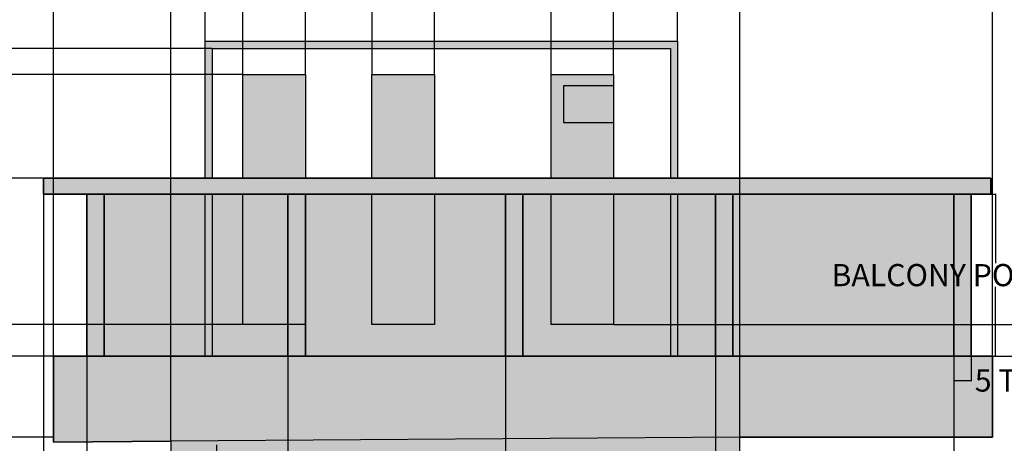
# Model space of a CAD drawing. Units: inches. Extents: x -655 to 499, y 20 to 616.
# Tile 3 of 7: x -409 to -137, y 248 to 365. Entities that reach past the tile are written whole.
import ezdxf

# ---------------------------------------------------------------- set-up
doc = ezdxf.new("R2010")
doc.units = ezdxf.units.IN
doc.header["$MEASUREMENT"] = 0
for name, color, linetype, lineweight in [('A-ANNO-DIMS', 2, 'Continuous', 18), ('A-ELEV', 7, 'Continuous', 35), ('A-ELEV-PATT', 9, 'Continuous', 13), ('A-GLAZ', 3, 'Continuous', 25)]:
    doc.layers.add(name, color=color, linetype=linetype, lineweight=lineweight)
doc.styles.get("Standard").update_dxf_attribs({"font": 'arial.ttf'})
doc.dimstyles.get("Standard").update_dxf_attribs({"dimtxt": 6.125, "dimasz": 0.18, "dimexe": 0.18, "dimexo": 0.0625, "dimgap": 0.09, "dimtad": 0, "dimtih": 1, "dimtoh": 1, "dimdec": 4, "dimzin": 0, "dimdsep": 46, "dimlunit": 4, "dimtxsty": 'Standard', "dimcen": 0.09, "dimadec": 0, "dimazin": 0, "dimtfac": 1, "dimtdec": 4, "dimtofl": 0, "dimtmove": 0, "dimatfit": 3, "dimfxl": 1, "dimtolj": 1, "dimtzin": 0, "dimarcsym": 0})

# ---------------------------------------------------------------- blocks, each defined once
blk = doc.blocks.new('BALCONY-POST')
for p, q in [((0, 0), (0, 44.79)), ((0, 44.79), (0, 44.79)), ((0, 44.79), (4.81, 44.79)), ((4.81, 44.79), (4.81, 0))]:
    blk.add_line(p, q)
blk = doc.blocks.new('*D4')
at = {"layer": 'A-ANNO-DIMS', "color": 0, "lineweight": -2, "transparency": 16777216}
for p, q in [((-145.9, 317.05), (-139.06, 317.05)), ((-139.24, 316.87), (-139.24, 297.92)), ((-139.24, 272.44), (-139.24, 291.4)), ((-145.9, 272.26), (-139.06, 272.26))]:
    blk.add_line(p, q, dxfattribs=at)
at = {"layer": 'A-ANNO-DIMS', "color": 0, "transparency": 16777216}
for points in [[(-139.27, 316.87), (-139.21, 316.87), (-139.24, 317.05)], [(-139.27, 272.44), (-139.21, 272.44), (-139.24, 272.26)]]:
    blk.add_solid(points, dxfattribs=at)
at = {"layer": 'Defpoints', "color": 0, "transparency": 16777216}
for p in [(-145.96, 317.05), (-139.24, 317.05), (-145.96, 272.26)]:
    blk.add_point(p, dxfattribs=at)
at = {"layer": 'A-ANNO-DIMS', "color": 0, "transparency": 16777216, "insert": (-139.24, 294.66), "char_height": 6.125, "attachment_point": 5}
blk.add_mtext('\\A1;BALCONY POST 45 TYP.', dxfattribs=at)
blk = doc.blocks.new('*D5')
at = {"layer": 'A-ANNO-DIMS', "color": 0, "lineweight": -2, "transparency": 16777216}
for p, q in [((-150.77, 272.2), (-150.77, 265.36)), ((-145.96, 272.2), (-145.96, 265.36)), ((-150.59, 265.54), (-146.14, 265.54)), ((-145.96, 265.54), (-145.78, 265.54))]:
    blk.add_line(p, q, dxfattribs=at)
at = {"layer": 'A-ANNO-DIMS', "color": 0, "transparency": 16777216}
for points in [[(-150.59, 265.57), (-150.59, 265.51), (-150.77, 265.54)], [(-146.14, 265.57), (-146.14, 265.51), (-145.96, 265.54)]]:
    blk.add_solid(points, dxfattribs=at)
at = {"layer": 'Defpoints', "color": 0, "transparency": 16777216}
for p in [(-150.77, 272.26), (-145.96, 272.26), (-145.96, 265.54)]:
    blk.add_point(p, dxfattribs=at)
at = {"layer": 'A-ANNO-DIMS', "color": 0, "transparency": 16777216, "insert": (-133.16, 265.54), "char_height": 6.125, "attachment_point": 5}
blk.add_mtext('\\A1;5 TYP.', dxfattribs=at)
blk = doc.blocks.new('*D10')
at = {"layer": 'A-ANNO-DIMS', "color": 0, "lineweight": -2, "transparency": 16777216}
for p, q in [((434.11, 393.11), (434.11, 23.7)), ((-590.16, 75.57), (-590.16, 23.7)), ((-589.98, 23.88), (-90.54, 23.88)), ((433.93, 23.88), (-65.51, 23.88))]:
    blk.add_line(p, q, dxfattribs=at)
at = {"layer": 'A-ANNO-DIMS', "color": 0, "transparency": 16777216}
for points in [[(-589.98, 23.91), (-589.98, 23.85), (-590.16, 23.88)], [(433.93, 23.91), (433.93, 23.85), (434.11, 23.88)]]:
    blk.add_solid(points, dxfattribs=at)
at = {"layer": 'Defpoints', "color": 0, "transparency": 16777216}
for p in [(434.11, 393.17), (-590.16, 75.63), (434.11, 23.88)]:
    blk.add_point(p, dxfattribs=at)
at = {"layer": 'A-ANNO-DIMS', "color": 0, "transparency": 16777216, "insert": (-78.02, 23.88), "char_height": 6.125, "attachment_point": 5}
blk.add_mtext('\\A1;1024.3', dxfattribs=at)
blk = doc.blocks.new('*D17')
at = {"layer": 'A-ANNO-DIMS', "color": 0, "lineweight": -2, "transparency": 16777216}
for p, q in [((-399.38, 249.9), (-399.38, 611.71)), ((-399.2, 611.53), (-282.57, 611.53)), ((-140.23, 611.53), (-256.86, 611.53)), ((-140.05, 249.9), (-140.05, 611.71))]:
    blk.add_line(p, q, dxfattribs=at)
at = {"layer": 'A-ANNO-DIMS', "color": 0, "transparency": 16777216}
for points in [[(-399.2, 611.56), (-399.2, 611.5), (-399.38, 611.53)], [(-140.23, 611.56), (-140.23, 611.5), (-140.05, 611.53)]]:
    blk.add_solid(points, dxfattribs=at)
at = {"layer": 'Defpoints', "color": 0, "transparency": 16777216}
for p in [(-140.05, 611.53), (-399.38, 249.84), (-140.05, 249.84)]:
    blk.add_point(p, dxfattribs=at)
at = {"layer": 'A-ANNO-DIMS', "color": 0, "transparency": 16777216, "insert": (-269.71, 611.53), "char_height": 6.125, "attachment_point": 5}
blk.add_mtext('\\A1;259.33', dxfattribs=at)
blk = doc.blocks.new('*D21')
at = {"layer": 'A-ANNO-DIMS', "color": 0, "lineweight": -2, "transparency": 16777216}
for p, q in [((179.11, 559.78), (486.04, 559.78)), ((485.86, 559.6), (485.86, 320.92)), ((485.86, 75.81), (485.86, 314.49)), ((-590.1, 75.63), (486.04, 75.63))]:
    blk.add_line(p, q, dxfattribs=at)
at = {"layer": 'A-ANNO-DIMS', "color": 0, "transparency": 16777216}
for points in [[(485.83, 559.6), (485.89, 559.6), (485.86, 559.78)], [(485.83, 75.81), (485.89, 75.81), (485.86, 75.63)]]:
    blk.add_solid(points, dxfattribs=at)
at = {"layer": 'Defpoints', "color": 0, "transparency": 16777216}
for p in [(179.05, 559.78), (485.86, 559.78), (-590.16, 75.63)]:
    blk.add_point(p, dxfattribs=at)
at = {"layer": 'A-ANNO-DIMS', "color": 0, "transparency": 16777216, "insert": (485.86, 317.7), "char_height": 6.125, "attachment_point": 5}
blk.add_mtext('\\A1;484.15', dxfattribs=at)
blk = doc.blocks.new('*D25')
at = {"layer": 'A-ANNO-DIMS', "color": 0, "lineweight": -2, "transparency": 16777216}
for p, q in [((-399.44, 249.84), (-642.09, 249.84)), ((-641.91, 249.66), (-641.91, 177.41)), ((-641.91, 98.71), (-641.91, 170.97)), ((-367.01, 98.53), (-642.09, 98.53))]:
    blk.add_line(p, q, dxfattribs=at)
at = {"layer": 'A-ANNO-DIMS', "color": 0, "transparency": 16777216}
for points in [[(-641.94, 249.66), (-641.88, 249.66), (-641.91, 249.84)], [(-641.94, 98.71), (-641.88, 98.71), (-641.91, 98.53)]]:
    blk.add_solid(points, dxfattribs=at)
at = {"layer": 'Defpoints', "color": 0, "transparency": 16777216}
for p in [(-399.38, 249.84), (-641.91, 98.53), (-366.94, 98.53)]:
    blk.add_point(p, dxfattribs=at)
at = {"layer": 'A-ANNO-DIMS', "color": 0, "transparency": 16777216, "insert": (-641.91, 174.19), "char_height": 6.125, "attachment_point": 5}
blk.add_mtext('\\A1;151.3', dxfattribs=at)
blk = doc.blocks.new('*D26')
at = {"layer": 'A-ANNO-DIMS', "color": 0, "lineweight": -2, "transparency": 16777216}
for p, q in [((-355.49, 357.29), (-642.09, 357.29)), ((-641.91, 357.11), (-641.91, 317.99)), ((-641.91, 272.44), (-641.91, 311.56)), ((-355.49, 272.26), (-642.09, 272.26))]:
    blk.add_line(p, q, dxfattribs=at)
at = {"layer": 'A-ANNO-DIMS', "color": 0, "transparency": 16777216}
for points in [[(-641.94, 357.11), (-641.88, 357.11), (-641.91, 357.29)], [(-641.94, 272.44), (-641.88, 272.44), (-641.91, 272.26)]]:
    blk.add_solid(points, dxfattribs=at)
at = {"layer": 'Defpoints', "color": 0, "transparency": 16777216}
for p in [(-641.91, 357.29), (-355.43, 357.29), (-355.43, 272.26)]:
    blk.add_point(p, dxfattribs=at)
at = {"layer": 'A-ANNO-DIMS', "color": 0, "transparency": 16777216, "insert": (-641.91, 314.77), "char_height": 6.125, "attachment_point": 5}
blk.add_mtext('\\A1;85.02', dxfattribs=at)
blk = doc.blocks.new('*D27')
at = {"layer": 'A-ANNO-DIMS', "color": 0, "lineweight": -2, "transparency": 16777216}
for p, q in [((-357.43, 359.35), (-357.43, 611.71)), ((-357.25, 611.53), (-347.21, 611.53)), ((-347.03, 350.2), (-347.03, 611.71)), ((-347.03, 611.53), (-346.85, 611.53))]:
    blk.add_line(p, q, dxfattribs=at)
at = {"layer": 'A-ANNO-DIMS', "color": 0, "transparency": 16777216}
for points in [[(-357.25, 611.56), (-357.25, 611.5), (-357.43, 611.53)], [(-347.21, 611.56), (-347.21, 611.5), (-347.03, 611.53)]]:
    blk.add_solid(points, dxfattribs=at)
at = {"layer": 'Defpoints', "color": 0, "transparency": 16777216}
for p in [(-347.03, 611.53), (-357.43, 359.29), (-347.03, 350.13)]:
    blk.add_point(p, dxfattribs=at)
at = {"layer": 'A-ANNO-DIMS', "color": 0, "transparency": 16777216, "insert": (-334.32, 611.53), "char_height": 6.125, "attachment_point": 5}
blk.add_mtext('\\A1;10.395', dxfattribs=at)
blk = doc.blocks.new('*D28')
at = {"layer": 'A-ANNO-DIMS', "color": 0, "lineweight": -2, "transparency": 16777216}
for p, q in [((-347.03, 350.2), (-347.03, 611.71)), ((-346.85, 611.53), (-329.96, 611.53)), ((-329.78, 350.2), (-329.78, 611.71)), ((-329.78, 611.53), (-329.6, 611.53))]:
    blk.add_line(p, q, dxfattribs=at)
at = {"layer": 'A-ANNO-DIMS', "color": 0, "transparency": 16777216}
for points in [[(-346.85, 611.56), (-346.85, 611.5), (-347.03, 611.53)], [(-329.96, 611.56), (-329.96, 611.5), (-329.78, 611.53)]]:
    blk.add_solid(points, dxfattribs=at)
at = {"layer": 'Defpoints', "color": 0, "transparency": 16777216}
for p in [(-329.78, 611.53), (-347.03, 350.13), (-329.78, 350.13)]:
    blk.add_point(p, dxfattribs=at)
at = {"layer": 'A-ANNO-DIMS', "color": 0, "transparency": 16777216, "insert": (-319.44, 611.53), "char_height": 6.125, "attachment_point": 5}
blk.add_mtext('\\A1;17.25', dxfattribs=at)
blk = doc.blocks.new('*D29')
at = {"layer": 'A-ANNO-DIMS', "color": 0, "lineweight": -2, "transparency": 16777216}
for p, q in [((-329.78, 350.2), (-329.78, 611.71)), ((-329.6, 611.53), (-311.57, 611.53)), ((-311.39, 350.2), (-311.39, 611.71)), ((-311.39, 611.53), (-311.21, 611.53))]:
    blk.add_line(p, q, dxfattribs=at)
at = {"layer": 'A-ANNO-DIMS', "color": 0, "transparency": 16777216}
for points in [[(-329.6, 611.56), (-329.6, 611.5), (-329.78, 611.53)], [(-311.57, 611.56), (-311.57, 611.5), (-311.39, 611.53)]]:
    blk.add_solid(points, dxfattribs=at)
at = {"layer": 'Defpoints', "color": 0, "transparency": 16777216}
for p in [(-311.39, 611.53), (-329.78, 350.13), (-311.39, 350.13)]:
    blk.add_point(p, dxfattribs=at)
at = {"layer": 'A-ANNO-DIMS', "color": 0, "transparency": 16777216, "insert": (-298.73, 611.53), "char_height": 6.125, "attachment_point": 5}
blk.add_mtext('\\A1;18.392', dxfattribs=at)
blk = doc.blocks.new('*D30')
at = {"layer": 'A-ANNO-DIMS', "color": 0, "lineweight": -2, "transparency": 16777216}
for p, q in [((-311.39, 350.2), (-311.39, 611.71)), ((-311.21, 611.53), (-294.32, 611.53)), ((-294.14, 350.2), (-294.14, 611.71)), ((-294.14, 611.53), (-293.96, 611.53))]:
    blk.add_line(p, q, dxfattribs=at)
at = {"layer": 'A-ANNO-DIMS', "color": 0, "transparency": 16777216}
for points in [[(-311.21, 611.56), (-311.21, 611.5), (-311.39, 611.53)], [(-294.32, 611.56), (-294.32, 611.5), (-294.14, 611.53)]]:
    blk.add_solid(points, dxfattribs=at)
at = {"layer": 'Defpoints', "color": 0, "transparency": 16777216}
for p in [(-294.14, 611.53), (-311.39, 350.13), (-294.14, 350.13)]:
    blk.add_point(p, dxfattribs=at)
at = {"layer": 'A-ANNO-DIMS', "color": 0, "transparency": 16777216, "insert": (-283.8, 611.53), "char_height": 6.125, "attachment_point": 5}
blk.add_mtext('\\A1;17.25', dxfattribs=at)
blk = doc.blocks.new('*D31')
at = {"layer": 'A-ANNO-DIMS', "color": 0, "lineweight": -2, "transparency": 16777216}
for p, q in [((-294.14, 350.2), (-294.14, 611.71)), ((-293.96, 611.53), (-290.86, 611.53)), ((-262.12, 611.53), (-265.21, 611.53)), ((-261.94, 350.2), (-261.94, 611.71))]:
    blk.add_line(p, q, dxfattribs=at)
at = {"layer": 'A-ANNO-DIMS', "color": 0, "transparency": 16777216}
for points in [[(-293.96, 611.56), (-293.96, 611.5), (-294.14, 611.53)], [(-262.12, 611.56), (-262.12, 611.5), (-261.94, 611.53)]]:
    blk.add_solid(points, dxfattribs=at)
at = {"layer": 'Defpoints', "color": 0, "transparency": 16777216}
for p in [(-261.94, 611.53), (-294.14, 350.13), (-261.94, 350.13)]:
    blk.add_point(p, dxfattribs=at)
at = {"layer": 'A-ANNO-DIMS', "color": 0, "transparency": 16777216, "insert": (-278.04, 611.53), "char_height": 6.125, "attachment_point": 5}
blk.add_mtext('\\A1;32.205', dxfattribs=at)
blk = doc.blocks.new('*D32')
at = {"layer": 'A-ANNO-DIMS', "color": 0, "lineweight": -2, "transparency": 16777216}
for p, q in [((-261.94, 350.2), (-261.94, 611.71)), ((-261.76, 611.53), (-244.87, 611.53)), ((-244.69, 350.2), (-244.69, 611.71)), ((-244.69, 611.53), (-244.51, 611.53))]:
    blk.add_line(p, q, dxfattribs=at)
at = {"layer": 'A-ANNO-DIMS', "color": 0, "transparency": 16777216}
for points in [[(-261.76, 611.56), (-261.76, 611.5), (-261.94, 611.53)], [(-244.87, 611.56), (-244.87, 611.5), (-244.69, 611.53)]]:
    blk.add_solid(points, dxfattribs=at)
at = {"layer": 'Defpoints', "color": 0, "transparency": 16777216}
for p in [(-244.69, 611.53), (-261.94, 350.13), (-244.69, 350.13)]:
    blk.add_point(p, dxfattribs=at)
at = {"layer": 'A-ANNO-DIMS', "color": 0, "transparency": 16777216, "insert": (-234.35, 611.53), "char_height": 6.125, "attachment_point": 5}
blk.add_mtext('\\A1;17.25', dxfattribs=at)
blk = doc.blocks.new('*D33')
at = {"layer": 'A-ANNO-DIMS', "color": 0, "lineweight": -2, "transparency": 16777216}
for p, q in [((-244.69, 350.2), (-244.69, 611.71)), ((-244.51, 611.53), (-227.19, 611.53)), ((-227.01, 359.35), (-227.01, 611.71)), ((-227.01, 611.53), (-226.83, 611.53))]:
    blk.add_line(p, q, dxfattribs=at)
at = {"layer": 'A-ANNO-DIMS', "color": 0, "transparency": 16777216}
for points in [[(-244.51, 611.56), (-244.51, 611.5), (-244.69, 611.53)], [(-227.19, 611.56), (-227.19, 611.5), (-227.01, 611.53)]]:
    blk.add_solid(points, dxfattribs=at)
at = {"layer": 'Defpoints', "color": 0, "transparency": 16777216}
for p in [(-227.01, 611.53), (-227.01, 359.29), (-244.69, 350.13)]:
    blk.add_point(p, dxfattribs=at)
at = {"layer": 'A-ANNO-DIMS', "color": 0, "transparency": 16777216, "insert": (-214.31, 611.53), "char_height": 6.125, "attachment_point": 5}
blk.add_mtext('\\A1;17.677', dxfattribs=at)
blk = doc.blocks.new('*D34')
at = {"layer": 'A-ANNO-DIMS', "color": 0, "lineweight": -2, "transparency": 16777216}
for p, q in [((-347.1, 350.13), (-642.09, 350.13)), ((-641.91, 349.95), (-641.91, 318.77)), ((-641.91, 281.15), (-641.91, 312.33)), ((-347.1, 280.97), (-642.09, 280.97))]:
    blk.add_line(p, q, dxfattribs=at)
at = {"layer": 'A-ANNO-DIMS', "color": 0, "transparency": 16777216}
for points in [[(-641.94, 349.95), (-641.88, 349.95), (-641.91, 350.13)], [(-641.94, 281.15), (-641.88, 281.15), (-641.91, 280.97)]]:
    blk.add_solid(points, dxfattribs=at)
at = {"layer": 'Defpoints', "color": 0, "transparency": 16777216}
for p in [(-347.03, 350.13), (-641.91, 280.97), (-347.03, 280.97)]:
    blk.add_point(p, dxfattribs=at)
at = {"layer": 'A-ANNO-DIMS', "color": 0, "transparency": 16777216, "insert": (-641.91, 315.55), "char_height": 6.125, "attachment_point": 5}
blk.add_mtext('\\A1;69.17', dxfattribs=at)
blk = doc.blocks.new('*D35')
at = {"layer": 'A-ANNO-DIMS', "color": 0, "lineweight": -2, "transparency": 16777216}
for p, q in [((-244.62, 280.97), (486.04, 280.97)), ((485.86, 280.79), (485.86, 279.83)), ((-226.95, 272.26), (486.04, 272.26)), ((485.86, 272.44), (485.86, 273.4))]:
    blk.add_line(p, q, dxfattribs=at)
at = {"layer": 'A-ANNO-DIMS', "color": 0, "transparency": 16777216}
for points in [[(485.83, 280.79), (485.89, 280.79), (485.86, 280.97)], [(485.83, 272.44), (485.89, 272.44), (485.86, 272.26)]]:
    blk.add_solid(points, dxfattribs=at)
at = {"layer": 'Defpoints', "color": 0, "transparency": 16777216}
for p in [(-244.69, 280.97), (-227.01, 272.26), (485.86, 272.26)]:
    blk.add_point(p, dxfattribs=at)
at = {"layer": 'A-ANNO-DIMS', "color": 0, "transparency": 16777216, "insert": (485.86, 276.61), "char_height": 6.125, "attachment_point": 5}
blk.add_mtext('\\A1;8.706', dxfattribs=at)
blk = doc.blocks.new('*D36')
at = {"layer": 'A-ANNO-DIMS', "color": 0, "lineweight": -2, "transparency": 16777216}
for p, q in [((-399.44, 272.26), (-642.09, 272.26)), ((-641.91, 272.08), (-641.91, 264.22)), ((-641.91, 250.02), (-641.91, 257.89)), ((-399.44, 249.84), (-642.09, 249.84))]:
    blk.add_line(p, q, dxfattribs=at)
at = {"layer": 'A-ANNO-DIMS', "color": 0, "transparency": 16777216}
for points in [[(-641.94, 272.08), (-641.88, 272.08), (-641.91, 272.26)], [(-641.94, 250.02), (-641.88, 250.02), (-641.91, 249.84)]]:
    blk.add_solid(points, dxfattribs=at)
at = {"layer": 'Defpoints', "color": 0, "transparency": 16777216}
for p in [(-641.91, 272.26), (-399.38, 272.26), (-399.38, 249.84)]:
    blk.add_point(p, dxfattribs=at)
at = {"layer": 'A-ANNO-DIMS', "color": 0, "transparency": 16777216, "insert": (-641.91, 261.05), "char_height": 6.125, "attachment_point": 5}
blk.add_mtext('\\A1;22.42', dxfattribs=at)
blk = doc.blocks.new('*D37')
at = {"layer": 'A-ANNO-DIMS', "color": 0, "lineweight": -2, "transparency": 16777216}
for p, q in [((-402.14, 321.49), (-642.09, 321.49)), ((-641.91, 321.31), (-641.91, 300.09)), ((-641.91, 272.44), (-641.91, 293.66)), ((-399.44, 272.26), (-642.09, 272.26))]:
    blk.add_line(p, q, dxfattribs=at)
at = {"layer": 'A-ANNO-DIMS', "color": 0, "transparency": 16777216}
for points in [[(-641.94, 321.31), (-641.88, 321.31), (-641.91, 321.49)], [(-641.94, 272.44), (-641.88, 272.44), (-641.91, 272.26)]]:
    blk.add_solid(points, dxfattribs=at)
at = {"layer": 'Defpoints', "color": 0, "transparency": 16777216}
for p in [(-641.91, 321.49), (-402.07, 321.49), (-399.38, 272.26)]:
    blk.add_point(p, dxfattribs=at)
at = {"layer": 'A-ANNO-DIMS', "color": 0, "transparency": 16777216, "insert": (-641.91, 296.87), "char_height": 6.125, "attachment_point": 5}
blk.add_mtext('\\A1;49.22', dxfattribs=at)
blk = doc.blocks.new('*D38')
at = {"layer": 'A-ANNO-DIMS', "color": 0, "lineweight": -2, "transparency": 16777216}
for p, q in [((-402.07, 316.99), (-402.07, 23.7)), ((-390.18, 316.99), (-390.18, 23.7)), ((-401.89, 23.88), (-390.36, 23.88)), ((-390.18, 23.88), (-390, 23.88))]:
    blk.add_line(p, q, dxfattribs=at)
at = {"layer": 'A-ANNO-DIMS', "color": 0, "transparency": 16777216}
for points in [[(-401.89, 23.91), (-401.89, 23.85), (-402.07, 23.88)], [(-390.36, 23.91), (-390.36, 23.85), (-390.18, 23.88)]]:
    blk.add_solid(points, dxfattribs=at)
at = {"layer": 'Defpoints', "color": 0, "transparency": 16777216}
for p in [(-402.07, 317.05), (-390.18, 317.05), (-390.18, 23.88)]:
    blk.add_point(p, dxfattribs=at)
at = {"layer": 'A-ANNO-DIMS', "color": 0, "transparency": 16777216, "insert": (-377.47, 23.88), "char_height": 6.125, "attachment_point": 5}
blk.add_mtext('\\A1;11.898', dxfattribs=at)
blk = doc.blocks.new('*D39')
at = {"layer": 'A-ANNO-DIMS', "color": 0, "lineweight": -2, "transparency": 16777216}
for p, q in [((-390.18, 316.99), (-390.18, 23.7)), ((-334.6, 316.99), (-334.6, 23.7)), ((-390, 23.88), (-372.82, 23.88)), ((-334.78, 23.88), (-351.96, 23.88))]:
    blk.add_line(p, q, dxfattribs=at)
at = {"layer": 'A-ANNO-DIMS', "color": 0, "transparency": 16777216}
for points in [[(-390, 23.91), (-390, 23.85), (-390.18, 23.88)], [(-334.78, 23.91), (-334.78, 23.85), (-334.6, 23.88)]]:
    blk.add_solid(points, dxfattribs=at)
at = {"layer": 'Defpoints', "color": 0, "transparency": 16777216}
for p in [(-390.18, 317.05), (-334.6, 317.05), (-334.6, 23.88)]:
    blk.add_point(p, dxfattribs=at)
at = {"layer": 'A-ANNO-DIMS', "color": 0, "transparency": 16777216, "insert": (-362.39, 23.88), "char_height": 6.125, "attachment_point": 5}
blk.add_mtext('\\A1;55.58', dxfattribs=at)
blk = doc.blocks.new('*D40')
at = {"layer": 'A-ANNO-DIMS', "color": 0, "lineweight": -2, "transparency": 16777216}
for p, q in [((-334.6, 316.99), (-334.6, 23.7)), ((-274.52, 316.99), (-274.52, 23.7)), ((-334.42, 23.88), (-315, 23.88)), ((-274.7, 23.88), (-294.12, 23.88))]:
    blk.add_line(p, q, dxfattribs=at)
at = {"layer": 'A-ANNO-DIMS', "color": 0, "transparency": 16777216}
for points in [[(-334.42, 23.91), (-334.42, 23.85), (-334.6, 23.88)], [(-274.7, 23.91), (-274.7, 23.85), (-274.52, 23.88)]]:
    blk.add_solid(points, dxfattribs=at)
at = {"layer": 'Defpoints', "color": 0, "transparency": 16777216}
for p in [(-334.6, 317.05), (-274.52, 317.05), (-274.52, 23.88)]:
    blk.add_point(p, dxfattribs=at)
at = {"layer": 'A-ANNO-DIMS', "color": 0, "transparency": 16777216, "insert": (-304.56, 23.88), "char_height": 6.125, "attachment_point": 5}
blk.add_mtext('\\A1;60.07', dxfattribs=at)
blk = doc.blocks.new('*D41')
at = {"layer": 'A-ANNO-DIMS', "color": 0, "lineweight": -2, "transparency": 16777216}
for p, q in [((-274.52, 316.99), (-274.52, 23.7)), ((-216.57, 316.99), (-216.57, 23.7)), ((-274.34, 23.88), (-256, 23.88)), ((-216.75, 23.88), (-235.1, 23.88))]:
    blk.add_line(p, q, dxfattribs=at)
at = {"layer": 'A-ANNO-DIMS', "color": 0, "transparency": 16777216}
for points in [[(-274.34, 23.91), (-274.34, 23.85), (-274.52, 23.88)], [(-216.75, 23.91), (-216.75, 23.85), (-216.57, 23.88)]]:
    blk.add_solid(points, dxfattribs=at)
at = {"layer": 'Defpoints', "color": 0, "transparency": 16777216}
for p in [(-274.52, 317.05), (-216.57, 317.05), (-216.57, 23.88)]:
    blk.add_point(p, dxfattribs=at)
at = {"layer": 'A-ANNO-DIMS', "color": 0, "transparency": 16777216, "insert": (-245.55, 23.88), "char_height": 6.125, "attachment_point": 5}
blk.add_mtext('\\A1;57.95', dxfattribs=at)
blk = doc.blocks.new('*D42')
at = {"layer": 'A-ANNO-DIMS', "color": 0, "lineweight": -2, "transparency": 16777216}
for p, q in [((-216.57, 316.99), (-216.57, 23.7)), ((-150.77, 316.99), (-150.77, 23.7)), ((-216.39, 23.88), (-191.74, 23.88)), ((-150.95, 23.88), (-175.6, 23.88))]:
    blk.add_line(p, q, dxfattribs=at)
at = {"layer": 'A-ANNO-DIMS', "color": 0, "transparency": 16777216}
for points in [[(-216.39, 23.91), (-216.39, 23.85), (-216.57, 23.88)], [(-150.95, 23.91), (-150.95, 23.85), (-150.77, 23.88)]]:
    blk.add_solid(points, dxfattribs=at)
at = {"layer": 'Defpoints', "color": 0, "transparency": 16777216}
for p in [(-216.57, 317.05), (-150.77, 317.05), (-150.77, 23.88)]:
    blk.add_point(p, dxfattribs=at)
at = {"layer": 'A-ANNO-DIMS', "color": 0, "transparency": 16777216, "insert": (-183.67, 23.88), "char_height": 6.125, "attachment_point": 5}
blk.add_mtext('\\A1;65.8', dxfattribs=at)
blk = doc.blocks.new('*D43')
at = {"layer": 'A-ANNO-DIMS', "color": 0, "lineweight": -2, "transparency": 16777216}
for p, q in [((-366.94, 248.81), (-366.94, 611.71)), ((-366.76, 611.53), (-300.88, 611.53)), ((-209.98, 611.53), (-275.87, 611.53)), ((-209.8, 99.69), (-209.8, 611.71))]:
    blk.add_line(p, q, dxfattribs=at)
at = {"layer": 'A-ANNO-DIMS', "color": 0, "transparency": 16777216}
for points in [[(-366.76, 611.56), (-366.76, 611.5), (-366.94, 611.53)], [(-209.98, 611.56), (-209.98, 611.5), (-209.8, 611.53)]]:
    blk.add_solid(points, dxfattribs=at)
at = {"layer": 'Defpoints', "color": 0, "transparency": 16777216}
for p in [(-209.8, 611.53), (-366.94, 248.74), (-209.8, 99.63)]:
    blk.add_point(p, dxfattribs=at)
at = {"layer": 'A-ANNO-DIMS', "color": 0, "transparency": 16777216, "insert": (-288.37, 611.53), "char_height": 6.125, "attachment_point": 5}
blk.add_mtext('\\A1;157.14', dxfattribs=at)
blk = doc.blocks.new('*D44')
at = {"layer": 'A-ANNO-DIMS', "color": 0, "lineweight": -2, "transparency": 16777216}
for p, q in [((-366.94, 248.68), (-366.94, 23.7)), ((-354.35, 247.78), (-354.35, 23.7)), ((-366.76, 23.88), (-354.53, 23.88)), ((-354.35, 23.88), (-354.17, 23.88))]:
    blk.add_line(p, q, dxfattribs=at)
at = {"layer": 'A-ANNO-DIMS', "color": 0, "transparency": 16777216}
for points in [[(-366.76, 23.91), (-366.76, 23.85), (-366.94, 23.88)], [(-354.53, 23.91), (-354.53, 23.85), (-354.35, 23.88)]]:
    blk.add_solid(points, dxfattribs=at)
at = {"layer": 'Defpoints', "color": 0, "transparency": 16777216}
for p in [(-366.94, 248.74), (-354.35, 247.84), (-354.35, 23.88)]:
    blk.add_point(p, dxfattribs=at)
at = {"layer": 'A-ANNO-DIMS', "color": 0, "transparency": 16777216, "insert": (-342.25, 23.88), "char_height": 6.125, "attachment_point": 5}
blk.add_mtext('\\A1;12.591', dxfattribs=at)

msp = doc.modelspace()

# ---------------------------------------------------------------- hatches: boundary and pattern name
at = {"layer": 'A-ELEV-PATT'}
h = msp.add_hatch(color=256, dxfattribs=at)
h.dxf.hatch_style = 1
h.paths.add_polyline_path([(-140.0489, 272.2618), (-399.3758, 272.2618), (-399.3758, 249.8418), (-399.3758, 248.5179), (-366.9446, 248.7444), (-209.8047, 249.8418), (-183.5755, 249.8418), (-140.0489, 249.8418)])
h.paths.add_polyline_path([(-211.7589, 317.0515), (-216.5713, 317.0515), (-216.5713, 272.2618), (-211.7589, 272.2618)])
h.paths.add_polyline_path([(-145.96, 317.0515), (-150.7725, 317.0515), (-150.7725, 272.2618), (-145.96, 272.2618)])
h.paths.add_polyline_path([(-140.5198, 321.4867), (-402.0739, 321.4867), (-402.0739, 317.0515), (-390.1757, 317.0515), (-385.3633, 317.0515), (-150.7725, 317.0515), (-145.96, 317.0515), (-140.5198, 317.0515)])
h.paths.add_polyline_path([(-269.7123, 317.0515), (-274.5248, 317.0515), (-274.5248, 272.2618), (-269.7123, 272.2618)])
h.paths.add_polyline_path([(-329.7837, 317.0515), (-334.5961, 317.0515), (-334.5961, 280.9678), (-329.7837, 280.9678)])
h.paths.add_polyline_path([(-329.7837, 280.9678), (-334.5961, 280.9678), (-334.5961, 272.2618), (-329.7837, 272.2618)])
h.paths.add_polyline_path([(-385.3633, 317.0515), (-390.1757, 317.0515), (-390.1757, 272.2618), (-385.3633, 272.2618)])
h.paths.add_polyline_path([(-229.0087, 240.4184), (-354.3532, 240.4184), (-354.2854, 210.6425), (-315.9956, 210.6425), (-315.9956, 210.9348), (-277.6793, 210.7995), (-277.6793, 210.6425), (-273.1052, 210.6425), (-273.1052, 210.7995), (-229.3637, 210.6425), (-229.0087, 210.6425)])
h.paths.add_polyline_path([(-229.0087, 145.8007), (-354.3532, 145.8007), (-354.3532, 101.6296), (-229.0087, 101.6296)])
h.paths.add_polyline_path([(-229.0087, 210.6425), (-229.3637, 210.6425), (-229.3637, 151.3385), (-273.1052, 151.4955), (-273.1052, 210.6425), (-277.6793, 210.6425), (-277.6793, 151.4955), (-315.9956, 151.6308), (-315.9956, 210.6425), (-318.9742, 210.6425), (-318.9742, 151.3385), (-354.3532, 151.3385), (-354.3532, 145.8007), (-229.0087, 145.8007)])
h.paths.add_polyline_path([(-229.0087, 247.8418), (-354.3532, 247.8418), (-354.3532, 240.4184), (-229.0087, 240.4184)])
h.paths.add_polyline_path([(4.4271, 93.6296), (-100.4134, 93.6296), (-124.8077, 93.6296), (-126.8077, 93.6296), (-126.8077, 87.6296), (4.4271, 87.6296)])
h.paths.add_polyline_path([(4.4271, 99.6296), (-100.4134, 99.6296), (-100.4134, 93.6296), (4.4271, 93.6296)])
h.paths.add_polyline_path([(99.4982, 99.6296), (6.4271, 99.6296), (6.4271, 93.6296), (99.4982, 93.6296)])
h.paths.add_polyline_path([(99.4982, 93.6296), (6.4271, 93.6296), (6.4271, 87.6296), (99.4982, 87.6296)])
h.paths.add_polyline_path([(304.2843, 311.436), (230.0144, 311.076), (230.0144, 282.9577), (270.6361, 282.9577), (304.4665, 273.8535)])
h.paths.add_polyline_path([(304.1054, 348.3371), (304.1054, 356.2861), (230.0144, 356.2861), (230.0144, 348.3443), (230.0144, 311.076), (304.2843, 311.436)])
h.paths.add_polyline_path([(255.5586, 316.5111), (255.5586, 350.0185), (275.6848, 350.0185), (275.6848, 316.5111)], flags=16)
h.paths.add_polyline_path([(278.0676, 316.5111), (278.0676, 350.0185), (301.4074, 350.0185), (301.4074, 316.5111)], flags=16)
h.paths.add_polyline_path([(253.2029, 316.5111), (233.8107, 316.5111), (233.8107, 350.0185), (253.2029, 350.0185)], flags=16)
h.paths.add_polyline_path([(179.0482, 559.7795), (153.2347, 535.8185), (165.0976, 535.8185), (192.9989, 535.8185), (201.2897, 535.8185)])
h.paths.add_polyline_path([(347.8163, 516.7932), (322.0028, 492.8322), (333.8657, 492.8322), (361.7669, 492.8322), (370.0577, 492.8322)])
h = msp.add_hatch(color=256, dxfattribs=at)
h.dxf.hatch_style = 1
h.paths.add_polyline_path([(-209.8047, 249.8418), (-366.9446, 248.7444), (-366.9446, 98.5321), (-209.8047, 99.6296)])
h.paths.add_polyline_path([(-229.0087, 101.6296), (-354.3532, 101.6296), (-354.3532, 247.8418), (-229.0087, 247.8418), (-229.0087, 240.4184), (-228.941, 210.6425), (-229.0087, 210.6425)], flags=16)
h.paths.add_polyline_path([(-229.3637, 151.3385), (-273.1052, 151.4955), (-273.1052, 210.7995), (-229.3637, 210.6425)], flags=0)
h.paths.add_polyline_path([(-277.6793, 151.4955), (-315.9956, 151.6308), (-315.9956, 210.9348), (-277.6793, 210.7995)], flags=0)
h.paths.add_polyline_path([(-318.9742, 151.3385), (-354.3532, 151.3385), (-354.3532, 210.6425), (-318.9742, 210.6425)], flags=0)
h.paths.add_polyline_path([(230.0144, 348.3443), (230.0144, 356.2861), (304.1054, 356.2861), (304.1054, 348.3371), (304.4665, 273.8535), (307.4704, 273.0451), (307.1054, 348.3443), (307.1054, 359.2861), (227.0144, 359.2861), (227.0144, 348.3443), (227.0144, 282.9577), (230.0144, 282.9577)])
h = msp.add_hatch(color=256, dxfattribs=at)
h.dxf.hatch_style = 1
h.paths.add_polyline_path([(-355.429, 357.2861), (-229.0087, 357.2861), (-229.0087, 321.4867), (-227.0087, 321.4867), (-227.0087, 359.2861), (-357.429, 359.2861), (-357.429, 321.4867), (-355.429, 321.4867)])
h.paths.add_polyline_path([(-355.429, 317.0515), (-357.429, 317.0515), (-357.429, 272.2618), (-355.429, 272.2618)])
h.paths.add_polyline_path([(-227.0087, 317.0515), (-229.0087, 317.0515), (-229.0087, 272.2618), (-227.0087, 272.2618)])
h = msp.add_hatch(color=256, dxfattribs=at)
h.dxf.hatch_style = 1
h.paths.add_polyline_path([(-329.7837, 350.1333), (-347.0336, 350.1333), (-347.0336, 321.4867), (-329.7837, 321.4867)])
h.paths.add_polyline_path([(-294.1413, 350.1333), (-311.3912, 350.1333), (-311.3912, 321.4867), (-294.1413, 321.4867)])
h.paths.add_polyline_path([(-294.1413, 317.0515), (-311.3912, 317.0515), (-311.3912, 280.9678), (-294.1413, 280.9678)])
h.paths.add_polyline_path([(-334.5961, 317.0515), (-347.0336, 317.0515), (-347.0336, 280.9678), (-334.5961, 280.9678)])
h.paths.add_polyline_path([(-244.6859, 336.719), (-258.4486, 336.719), (-258.4486, 347.0139), (-244.6859, 347.0139), (-244.6859, 350.1333), (-261.9358, 350.1333), (-261.9358, 321.4867), (-244.6859, 321.4867)])
h.paths.add_polyline_path([(-244.6859, 317.0515), (-261.9358, 317.0515), (-261.9358, 280.9678), (-244.6859, 280.9678)])
h.paths.add_polyline_path([(-244.6859, 347.0139), (-258.4486, 347.0139), (-258.4486, 336.719), (-244.6859, 336.719)], flags=17)
h.paths.add_polyline_path([(-318.9742, 210.6425), (-354.3532, 210.6425), (-354.3532, 151.3385), (-318.9742, 151.3385)])
h.paths.add_polyline_path([(-277.6793, 210.6425), (-315.9956, 210.6425), (-315.9956, 151.6308), (-277.6793, 151.4955)])
h.paths.add_polyline_path([(-229.3637, 210.6425), (-273.1052, 210.6425), (-273.1052, 151.4955), (-229.3637, 151.3385)])
h.paths.add_polyline_path([(-19.537, 192.4712), (-40.2951, 192.4712), (-40.2951, 150.3082), (-19.537, 150.3082)])
h.paths.add_polyline_path([(2.4271, 231.274), (-62.1158, 231.274), (-62.1158, 210.7923), (2.4271, 210.7923)])
h.paths.add_polyline_path([(72.97, 231.274), (8.4271, 231.274), (8.4271, 210.7923), (72.97, 210.7923)])
h.paths.add_polyline_path([(51.0059, 192.4712), (30.2478, 192.4712), (30.2478, 150.3082), (51.0059, 150.3082)])
h.paths.add_polyline_path([(51.0059, 132.6671), (30.2478, 132.6671), (30.2478, 112.5254), (51.0059, 112.5254)])
h.paths.add_polyline_path([(-19.537, 132.6671), (-40.2951, 132.6671), (-40.2951, 112.5254), (-19.537, 112.5254)])
h.paths.add_polyline_path([(275.6848, 350.0185), (255.5586, 350.0185), (255.5586, 316.5111), (275.6848, 316.5111)])
h.paths.add_polyline_path([(301.4074, 350.0185), (278.0676, 350.0185), (278.0676, 316.5111), (301.4074, 316.5111)])
h.paths.add_polyline_path([(253.2029, 350.0185), (233.8107, 350.0185), (233.8107, 316.5111), (253.2029, 316.5111)])
h = msp.add_hatch(color=256, dxfattribs=at)
h.dxf.hatch_style = 1
h.paths.add_polyline_path([(-150.7725, 317.0515), (-211.7589, 317.0515), (-211.7589, 272.2618), (-150.7725, 272.2618)])
h.paths.add_polyline_path([(-229.0087, 317.0515), (-244.6859, 317.0515), (-244.6859, 280.9678), (-261.9358, 280.9678), (-261.9358, 317.0515), (-269.7123, 317.0515), (-269.7123, 272.2618), (-229.0087, 272.2618)])
h.paths.add_polyline_path([(-216.5713, 317.0515), (-227.0087, 317.0515), (-227.0087, 272.2618), (-216.5713, 272.2618)])
h.paths.add_polyline_path([(-274.5248, 317.0515), (-294.1413, 317.0515), (-294.1413, 280.9678), (-311.3912, 280.9678), (-311.3912, 317.0515), (-329.7837, 317.0515), (-329.7837, 280.9678), (-329.7837, 272.2618), (-274.5248, 272.2618)])
h.paths.add_polyline_path([(-347.0336, 317.0515), (-355.429, 317.0515), (-355.429, 272.2618), (-334.5961, 272.2618), (-334.5961, 280.9678), (-347.0336, 280.9678)])
h.paths.add_polyline_path([(-357.429, 317.0515), (-385.3633, 317.0515), (-385.3633, 272.2618), (-357.429, 272.2618)])
h.paths.add_polyline_path([(176.2798, 243.6296), (109.2763, 243.6296), (109.2763, 194.9112), (176.2798, 194.9112)])
h.paths.add_polyline_path([(176.2798, 194.9112), (109.2763, 194.9112), (109.2763, 137.2003), (176.2798, 137.2003)])
h.paths.add_polyline_path([(236.7365, 243.6296), (176.2798, 243.6296), (176.2798, 194.9112), (236.7365, 194.9112)])
h.paths.add_polyline_path([(236.7365, 194.9112), (176.2798, 194.9112), (176.2798, 137.2003), (236.7365, 137.2003)])
h.paths.add_polyline_path([(236.7365, 137.2003), (176.2798, 137.2003), (176.2798, 99.6296), (236.7365, 99.6296)])
h.paths.add_polyline_path([(176.2798, 137.2003), (109.2763, 137.2003), (109.2763, 99.6296), (176.2798, 99.6296)])
h.paths.add_polyline_path([(301.3566, 137.2003), (236.7365, 137.2003), (236.7365, 99.6296), (301.3566, 99.6296)])
h.paths.add_polyline_path([(301.3566, 194.9112), (236.7365, 194.9112), (236.7365, 137.2003), (301.3566, 137.2003)])
h.paths.add_polyline_path([(301.3566, 243.6296), (236.7365, 243.6296), (236.7365, 194.9112), (301.3566, 194.9112)])
h.paths.add_polyline_path([(365.0401, 243.6296), (301.3566, 243.6296), (301.3566, 194.9112), (365.0401, 194.9112)])
h.paths.add_polyline_path([(365.0401, 194.9112), (301.3566, 194.9112), (301.3566, 137.2003), (365.0401, 137.2003)])
h.paths.add_polyline_path([(411.9901, 243.6296), (365.0401, 243.6296), (365.0401, 194.9112), (411.9901, 194.9112)])
h.paths.add_polyline_path([(411.9901, 194.9112), (365.0401, 194.9112), (365.0401, 99.6296), (411.9901, 99.6296)])
h.paths.add_polyline_path([(365.0401, 137.2003), (301.3566, 137.2003), (301.3566, 99.6296), (365.0401, 99.6296)])

# ---------------------------------------------------------------- linework, layer by layer
at = {"layer": 'A-ELEV'}
for p, q in [((-402.0739, 317.0515), (-402.0739, 321.4867)), ((-402.0739, 321.4867), (-140.5198, 321.4867)), ((-140.5198, 321.4867), (-140.5198, 317.0515)), ((-390.1757, 317.0515), (-402.0739, 317.0515)), ((-385.3633, 317.0515), (-150.7725, 317.0515)), ((-140.5198, 317.0515), (-145.96, 317.0515)), ((-140.5198, 317.0515), (-140.5198, 317.0515)), ((-140.0489, 272.2618), (-399.3758, 272.2618)), ((-399.3758, 272.2618), (-399.3758, 249.8418)), ((-140.0489, 249.8418), (-140.0489, 272.2618)), ((-399.3758, 248.5179), (-399.3758, 249.8418)), ((-366.9446, 248.7444), (-399.3758, 248.5179)), ((-209.8047, 249.8418), (-183.5755, 249.8418)), ((-183.5755, 249.8418), (-140.0489, 249.8418))]:
    msp.add_line(p, q, dxfattribs=at)
at = {"layer": 'A-GLAZ'}
for p, q in [((-357.429, 359.2861), (-227.0087, 359.2861)), ((-357.429, 321.4867), (-357.429, 359.2861)), ((-227.0087, 359.2861), (-227.0087, 321.4867)), ((-355.429, 357.2861), (-229.0087, 357.2861)), ((-355.429, 321.4867), (-355.429, 357.2861)), ((-229.0087, 357.2861), (-229.0087, 321.4867)), ((-357.429, 272.2618), (-357.429, 317.0515)), ((-355.429, 272.2618), (-355.429, 317.0515)), ((-229.0087, 317.0515), (-229.0087, 272.2618)), ((-227.0087, 317.0515), (-227.0087, 272.2618))]:
    msp.add_line(p, q, dxfattribs=at)
for points in [[(-347.0336, 321.4867), (-347.0336, 350.1333), (-329.7837, 350.1333), (-329.7837, 321.4867)], [(-311.3912, 321.4867), (-311.3912, 350.1333), (-294.1413, 350.1333), (-294.1413, 321.4867)], [(-261.9358, 321.4867), (-261.9358, 350.1333), (-244.6859, 350.1333), (-244.6859, 321.4867)], [(-329.7837, 317.0515), (-329.7837, 280.9678), (-347.0336, 280.9678), (-347.0336, 317.0515)], [(-294.1413, 317.0515), (-294.1413, 280.9678), (-311.3912, 280.9678), (-311.3912, 317.0515)], [(-244.6859, 317.0515), (-244.6859, 280.9678), (-261.9358, 280.9678), (-261.9358, 317.0515)]]:
    msp.add_lwpolyline(points, dxfattribs=at)
for points in [[(-258.4486, 347.0139), (-244.6859, 347.0139), (-244.6859, 336.719), (-258.4486, 336.719)], [(-366.9446, 98.5321), (-209.8047, 99.6296), (-209.8047, 249.8418), (-366.9446, 248.7444)]]:
    msp.add_lwpolyline(points, close=True, dxfattribs=at)

# ---------------------------------------------------------------- block references
at = {"layer": 'A-ELEV'}
for p in [(-390.176, 272.262), (-334.5965, 272.262), (-274.5251, 272.262), (-216.5716, 272.262), (-150.7728, 272.262)]:
    msp.add_blockref('BALCONY-POST', p, dxfattribs=at)

# ---------------------------------------------------------------- dimensions: what is measured, and where the dimension line sits
at = {"layer": 'A-ANNO-DIMS'}
for base, p1, p2, override, picture, middle in [((-140.0489, 611.5295), (-399.3758, 249.8418), (-140.0489, 249.8418), {"dimdec": 2, "dimlfac": 1, "dimrnd": 0, "dimzin": 0, "dimdsep": 46, "dimlunit": 2}, '*D17', (-269.7123, 611.5295)), ((-209.8047, 611.5295), (-366.9446, 248.7444), (-209.8047, 99.6296), {"dimdec": 2, "dimlfac": 1, "dimrnd": 0, "dimzin": 0, "dimdsep": 46, "dimlunit": 2}, '*D43', (-288.3746, 611.5295)), ((-347.0336, 611.5295), (-357.429, 359.2861), (-347.0336, 350.1333), {"dimdec": 3, "dimlfac": 1, "dimrnd": 0, "dimzin": 0, "dimdsep": 46, "dimlunit": 2}, '*D27', (-334.3152, 611.5295)), ((-329.7837, 611.5295), (-347.0336, 350.1333), (-329.7837, 350.1333), {"dimdec": 2, "dimlfac": 1, "dimrnd": 0, "dimzin": 0, "dimdsep": 46, "dimlunit": 2}, '*D28', (-319.4446, 611.5295)), ((-311.39124, 611.52951), (-329.78371, 350.13329), (-311.39124, 350.13329), {"dimdec": 3, "dimlfac": 1, "dimrnd": 0, "dimzin": 0, "dimdsep": 46, "dimlunit": 2}, '*D29', (-298.7271, 611.52951)), ((-294.1413, 611.5295), (-311.3912, 350.1333), (-294.1413, 350.1333), {"dimdec": 2, "dimlfac": 1, "dimrnd": 0, "dimzin": 0, "dimdsep": 46, "dimlunit": 2}, '*D30', (-283.8023, 611.5295)), ((-261.935835, 611.529514), (-294.141326, 350.133285), (-261.935835, 350.133285), {"dimdec": 3, "dimlfac": 1, "dimrnd": 0, "dimzin": 0, "dimdsep": 46, "dimlunit": 2}, '*D31', (-278.038581, 611.529514)), ((-244.6859, 611.5295), (-261.9358, 350.1333), (-244.6859, 350.1333), {"dimdec": 2, "dimlfac": 1, "dimrnd": 0, "dimzin": 0, "dimdsep": 46, "dimlunit": 2}, '*D32', (-234.3469, 611.5295)), ((-227.0087, 611.5295), (-244.6859, 350.1333), (-227.0087, 359.2861), {"dimdec": 3, "dimlfac": 1, "dimrnd": 0, "dimzin": 0, "dimdsep": 46, "dimlunit": 2}, '*D33', (-214.3132, 611.5295)), ((434.1137, 23.8796), (-590.1625, 75.6296), (434.1137, 393.1688), {"dimdec": 1, "dimlfac": 1, "dimrnd": 0, "dimzin": 0, "dimdsep": 46, "dimlunit": 2}, '*D10', (-78.0244, 23.8796)), ((-390.1757, 23.8796), (-402.0739, 317.0515), (-390.1757, 317.0515), {"dimdec": 3, "dimlfac": 1, "dimrnd": 0, "dimzin": 0, "dimdsep": 46, "dimlunit": 2}, '*D38', (-377.4739, 23.8796)), ((-334.5961, 23.8796), (-390.1757, 317.0515), (-334.5961, 317.0515), {"dimdec": 2, "dimlfac": 1, "dimrnd": 0, "dimzin": 0, "dimdsep": 46, "dimlunit": 2}, '*D39', (-362.3859, 23.8796)), ((-274.5248, 23.8796), (-334.5961, 317.0515), (-274.5248, 317.0515), {"dimdec": 2, "dimlfac": 1, "dimrnd": 0, "dimzin": 0, "dimdsep": 46, "dimlunit": 2}, '*D40', (-304.5605, 23.8796)), ((-216.5713, 23.8796), (-274.5248, 317.0515), (-216.5713, 317.0515), {"dimdec": 2, "dimlfac": 1, "dimrnd": 0, "dimzin": 0, "dimdsep": 46, "dimlunit": 2}, '*D41', (-245.548, 23.8796)), ((-150.7725, 23.8796), (-216.5713, 317.0515), (-150.7725, 317.0515), {"dimdec": 1, "dimlfac": 1, "dimrnd": 0, "dimzin": 0, "dimdsep": 46, "dimlunit": 2}, '*D42', (-183.6719, 23.8796)), ((-354.3532, 23.8796), (-366.9446, 248.7444), (-354.3532, 247.8418), {"dimdec": 3, "dimlfac": 1, "dimrnd": 0, "dimzin": 0, "dimdsep": 46, "dimlunit": 2}, '*D44', (-342.2489, 23.8796))]:
    dim = msp.add_linear_dim(base=base, p1=p1, p2=p2, dimstyle='Standard', override=override, dxfattribs=at)
    dim.commit()
    dim.dimension.update_dxf_attribs({"geometry": picture, "text_midpoint": middle})
for base, p1, p2, override, picture, middle in [((485.8637, 559.7795), (-590.1625, 75.6296), (179.0482, 559.7795), {"dimdec": 2, "dimlfac": 1, "dimrnd": 0, "dimzin": 0, "dimdsep": 46, "dimlunit": 2}, '*D21', (485.8637, 317.7046)), ((-641.9125, 357.2861), (-355.429, 272.2618), (-355.429, 357.2861), {"dimdec": 2, "dimlfac": 1, "dimrnd": 0, "dimzin": 0, "dimdsep": 46, "dimlunit": 2}, '*D26', (-641.9125, 314.7739)), ((-641.9125, 280.9678), (-347.0336, 350.1333), (-347.0336, 280.9678), {"dimdec": 2, "dimlfac": 1, "dimrnd": 0, "dimzin": 0, "dimdsep": 46, "dimlunit": 2}, '*D34', (-641.9125, 315.5506)), ((-641.9125, 321.4867), (-399.3758, 272.2618), (-402.0739, 321.4867), {"dimdec": 2, "dimlfac": 1, "dimrnd": 0, "dimzin": 0, "dimdsep": 46, "dimlunit": 2}, '*D37', (-641.9125, 296.8743)), ((485.8637, 272.2618), (-244.6859, 280.9678), (-227.0087, 272.2618), {"dimdec": 3, "dimlfac": 1, "dimrnd": 0, "dimzin": 0, "dimdsep": 46, "dimlunit": 2}, '*D35', (485.8637, 276.6148)), ((-641.9125, 272.2618), (-399.3758, 249.8418), (-399.3758, 272.2618), {"dimdec": 2, "dimlfac": 1, "dimrnd": 0, "dimzin": 0, "dimdsep": 46, "dimlunit": 2}, '*D36', (-641.9125, 261.0518)), ((-641.9125, 98.5321), (-399.3758, 249.8418), (-366.9446, 98.5321), {"dimdec": 1, "dimlfac": 1, "dimrnd": 0, "dimzin": 0, "dimdsep": 46, "dimlunit": 2}, '*D25', (-641.9125, 174.187))]:
    dim = msp.add_linear_dim(base=base, p1=p1, p2=p2, angle=90, dimstyle='Standard', override=override, dxfattribs=at)
    dim.commit()
    dim.dimension.update_dxf_attribs({"geometry": picture, "text_midpoint": middle})
dim = msp.add_linear_dim(base=(-139.2416, 317.0515), p1=(-145.96, 272.2618), p2=(-145.96, 317.0515), angle=90, text='BALCONY POST <> TYP.', dimstyle='Standard', override={"dimdec": 0, "dimlfac": 1, "dimrnd": 0, "dimzin": 0, "dimdsep": 46, "dimlunit": 2}, dxfattribs=at)
dim.commit()
dim.dimension.update_dxf_attribs({"geometry": '*D4', "text_midpoint": (-139.2416, 294.6566)})
dim = msp.add_linear_dim(base=(-145.96, 265.5434), p1=(-150.7725, 272.2618), p2=(-145.96, 272.2618), text='<> TYP.', dimstyle='Standard', override={"dimdec": 0, "dimlfac": 1, "dimrnd": 0, "dimzin": 0, "dimdsep": 46, "dimlunit": 2}, dxfattribs=at)
dim.commit()
dim.dimension.update_dxf_attribs({"geometry": '*D5', "text_midpoint": (-133.1622, 265.5434)})

doc.saveas('drawing.dxf')
